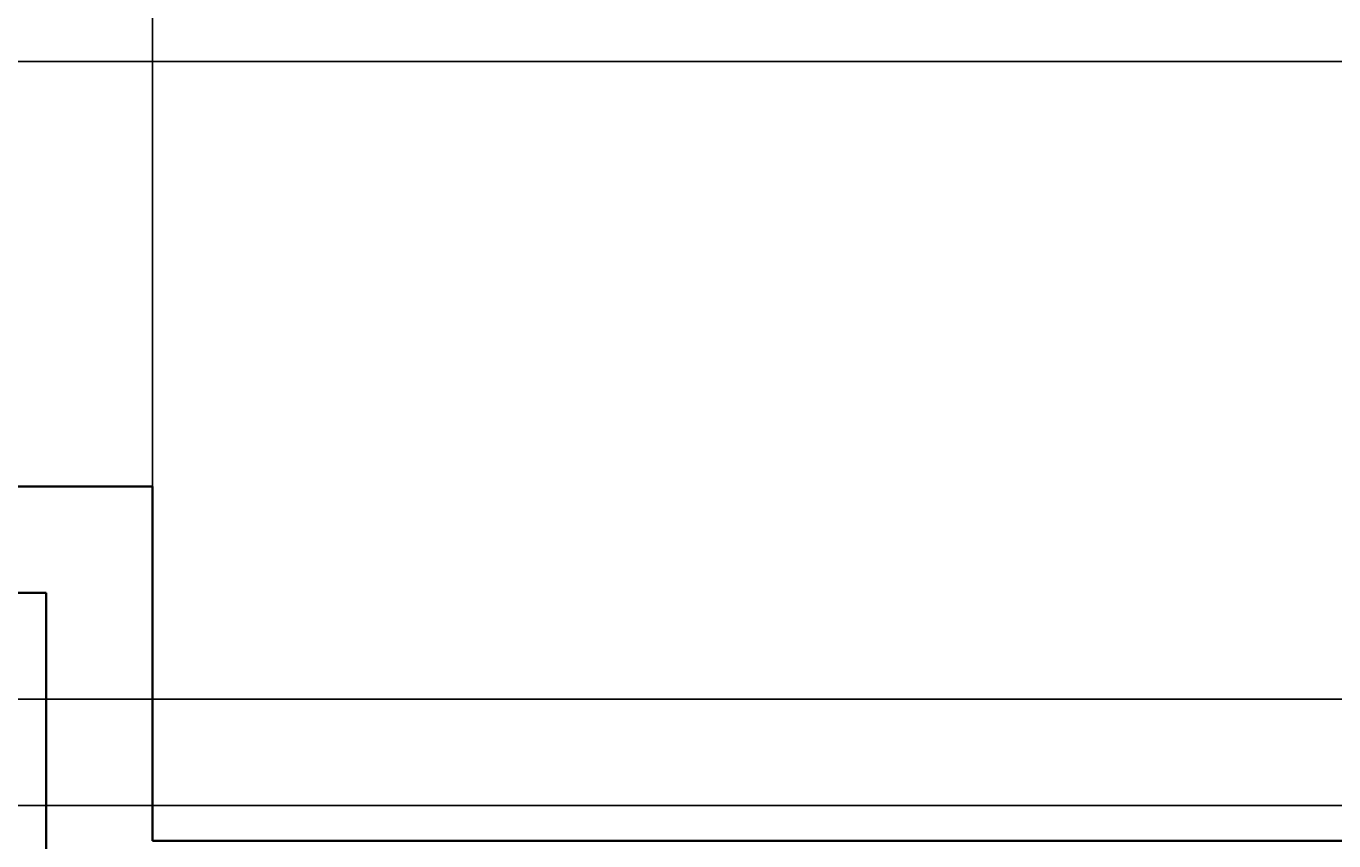
# Model space of a CAD drawing. Units: feet. Extents: x 105 to 1094, y -88 to 588.
# Tile 10 of 59: x 288 to 361, y 204 to 250. Entities that reach past the tile are written whole.
import ezdxf

# ---------------------------------------------------------------- set-up
doc = ezdxf.new("R2010")
doc.units = ezdxf.units.FT
doc.header["$MEASUREMENT"] = 0
doc.layers.add('A-ANNO-DIMS', color=2, linetype='Continuous', lineweight=18)
doc.layers.add('A-WALL', color=7, linetype='Continuous', lineweight=35)
doc.styles.get("Standard").update_dxf_attribs({"font": 'arial.ttf'})
doc.dimstyles.get("Standard").update_dxf_attribs({"dimtxt": 0.18, "dimasz": 0.18, "dimexe": 0.18, "dimexo": 0.0625, "dimgap": 0.09, "dimtad": 0, "dimtih": 1, "dimtoh": 1, "dimdec": 4, "dimzin": 0, "dimdsep": 46, "dimtxsty": 'Standard', "dimcen": 0.09, "dimadec": 0, "dimazin": 0, "dimtfac": 1, "dimtdec": 4, "dimtofl": 0, "dimtmove": 0, "dimatfit": 3, "dimfxl": 1, "dimtolj": 1, "dimtzin": 0, "dimarcsym": 0})

# ---------------------------------------------------------------- blocks, each defined once
blk = doc.blocks.new('*D20')
at = {"layer": 'A-ANNO-DIMS', "color": 0, "lineweight": -2, "transparency": 16777216}
for p, q in [((150.688, 276.019), (150.688, -88.149)), ((1048.688, 276.019), (1048.688, -88.149)), ((150.868, -87.969), (599.399, -87.969)), ((1048.508, -87.969), (599.977, -87.969))]:
    blk.add_line(p, q, dxfattribs=at)
at = {"layer": 'A-ANNO-DIMS', "color": 0, "transparency": 16777216}
for points in [[(150.868, -87.939), (150.868, -87.999), (150.688, -87.969)], [(1048.508, -87.939), (1048.508, -87.999), (1048.688, -87.969)]]:
    blk.add_solid(points, dxfattribs=at)
at = {"layer": 'Defpoints', "color": 0, "transparency": 16777216}
for p in [(150.688, 276.081), (1048.688, 276.081), (1048.688, -87.969)]:
    blk.add_point(p, dxfattribs=at)
at = {"layer": 'A-ANNO-DIMS', "color": 0, "transparency": 16777216, "insert": (599.688, -87.969), "char_height": 0.18, "attachment_point": 5}
blk.add_mtext('\\A1;898', dxfattribs=at)
blk = doc.blocks.new('*D21')
at = {"layer": 'A-ANNO-DIMS', "color": 0, "lineweight": -2, "transparency": 16777216}
for p, q in [((849.626, 543.081), (105.458, 543.081)), ((105.638, 542.901), (105.638, 250.263)), ((105.638, -42.739), (105.638, 249.899)), ((849.626, -42.919), (105.458, -42.919))]:
    blk.add_line(p, q, dxfattribs=at)
at = {"layer": 'A-ANNO-DIMS', "color": 0, "transparency": 16777216}
for points in [[(105.608, 542.901), (105.668, 542.901), (105.638, 543.081)], [(105.608, -42.739), (105.668, -42.739), (105.638, -42.919)]]:
    blk.add_solid(points, dxfattribs=at)
at = {"layer": 'Defpoints', "color": 0, "transparency": 16777216}
for p in [(105.638, 543.081), (849.688, 543.081), (849.688, -42.919)]:
    blk.add_point(p, dxfattribs=at)
at = {"layer": 'A-ANNO-DIMS', "color": 0, "transparency": 16777216, "insert": (105.638, 250.081), "char_height": 0.18, "attachment_point": 5}
blk.add_mtext('\\A1;586', dxfattribs=at)
blk = doc.blocks.new('*D36')
at = {"layer": 'A-ANNO-DIMS', "color": 0, "lineweight": -2, "transparency": 16777216}
for p, q in [((547.235, 248.081), (105.458, 248.081)), ((105.638, 247.901), (105.638, 230.263)), ((105.638, 212.261), (105.638, 229.899)), ((546.626, 212.081), (105.458, 212.081))]:
    blk.add_line(p, q, dxfattribs=at)
at = {"layer": 'A-ANNO-DIMS', "color": 0, "transparency": 16777216}
for points in [[(105.608, 247.901), (105.668, 247.901), (105.638, 248.081)], [(105.608, 212.261), (105.668, 212.261), (105.638, 212.081)]]:
    blk.add_solid(points, dxfattribs=at)
at = {"layer": 'Defpoints', "color": 0, "transparency": 16777216}
for p in [(105.638, 248.081), (547.298, 248.081), (546.688, 212.081)]:
    blk.add_point(p, dxfattribs=at)
at = {"layer": 'A-ANNO-DIMS', "color": 0, "transparency": 16777216, "insert": (105.638, 230.081), "char_height": 0.18, "attachment_point": 5}
blk.add_mtext('\\A1;36', dxfattribs=at)
blk = doc.blocks.new('*D38')
at = {"layer": 'A-ANNO-DIMS', "color": 0, "lineweight": -2, "transparency": 16777216}
for p, q in [((150.688, 224.144), (150.688, 588.311)), ((150.868, 588.131), (222.408, 588.131)), ((294.508, 588.131), (222.968, 588.131)), ((294.688, 224.144), (294.688, 588.311))]:
    blk.add_line(p, q, dxfattribs=at)
at = {"layer": 'A-ANNO-DIMS', "color": 0, "transparency": 16777216}
for points in [[(150.868, 588.161), (150.868, 588.101), (150.688, 588.131)], [(294.508, 588.161), (294.508, 588.101), (294.688, 588.131)]]:
    blk.add_solid(points, dxfattribs=at)
at = {"layer": 'Defpoints', "color": 0, "transparency": 16777216}
for p in [(294.688, 588.131), (150.688, 224.081), (294.688, 224.081)]:
    blk.add_point(p, dxfattribs=at)
at = {"layer": 'A-ANNO-DIMS', "color": 0, "transparency": 16777216, "insert": (222.688, 588.131), "char_height": 0.18, "attachment_point": 5}
blk.add_mtext('\\A1;144', dxfattribs=at)
blk = doc.blocks.new('*D39')
at = {"layer": 'A-ANNO-DIMS', "color": 0, "lineweight": -2, "transparency": 16777216}
for p, q in [((294.688, 204.144), (294.688, 588.311)), ((294.868, 588.131), (332.47, 588.131)), ((370.508, 588.131), (332.906, 588.131)), ((370.688, 204.144), (370.688, 588.311))]:
    blk.add_line(p, q, dxfattribs=at)
at = {"layer": 'A-ANNO-DIMS', "color": 0, "transparency": 16777216}
for points in [[(294.868, 588.161), (294.868, 588.101), (294.688, 588.131)], [(370.508, 588.161), (370.508, 588.101), (370.688, 588.131)]]:
    blk.add_solid(points, dxfattribs=at)
at = {"layer": 'Defpoints', "color": 0, "transparency": 16777216}
for p in [(370.688, 588.131), (294.688, 204.081), (370.688, 204.081)]:
    blk.add_point(p, dxfattribs=at)
at = {"layer": 'A-ANNO-DIMS', "color": 0, "transparency": 16777216, "insert": (332.688, 588.131), "char_height": 0.18, "attachment_point": 5}
blk.add_mtext('\\A1;76', dxfattribs=at)
blk = doc.blocks.new('*D46')
at = {"layer": 'A-ANNO-DIMS', "color": 0, "lineweight": -2, "transparency": 16777216}
for p, q in [((580.626, 206.081), (105.458, 206.081)), ((105.638, 205.901), (105.638, 173.263)), ((105.638, 140.261), (105.638, 172.899)), ((580.626, 140.081), (105.458, 140.081))]:
    blk.add_line(p, q, dxfattribs=at)
at = {"layer": 'A-ANNO-DIMS', "color": 0, "transparency": 16777216}
for points in [[(105.608, 205.901), (105.668, 205.901), (105.638, 206.081)], [(105.608, 140.261), (105.668, 140.261), (105.638, 140.081)]]:
    blk.add_solid(points, dxfattribs=at)
at = {"layer": 'Defpoints', "color": 0, "transparency": 16777216}
for p in [(580.688, 206.081), (105.638, 140.081), (580.688, 140.081)]:
    blk.add_point(p, dxfattribs=at)
at = {"layer": 'A-ANNO-DIMS', "color": 0, "transparency": 16777216, "insert": (105.638, 173.081), "char_height": 0.18, "attachment_point": 5}
blk.add_mtext('\\A1;66', dxfattribs=at)

msp = doc.modelspace()

# ---------------------------------------------------------------- linework, layer by layer
at = {"layer": 'A-WALL'}
for p, q in [((294.6883, 224.0812), (150.6883, 224.0812)), ((294.6883, 224.0812), (294.6883, 204.0812)), ((288.6883, 218.0812), (156.6883, 218.0812)), ((288.6883, 218.0812), (288.6883, 180.0812)), ((370.6883, 204.0812), (294.6883, 204.0812))]:
    msp.add_line(p, q, dxfattribs=at)

# ---------------------------------------------------------------- dimensions: what is measured, and where the dimension line sits
at = {"layer": 'A-ANNO-DIMS'}
for base, p1, p2, picture, middle in [((294.6883, 588.1312), (150.6883, 224.0812), (294.6883, 224.0812), '*D38', (222.6883, 588.1312)), ((370.6883, 588.1312), (294.6883, 204.0812), (370.6883, 204.0812), '*D39', (332.6883, 588.1312)), ((1048.6883, -87.9688), (150.6883, 276.0812), (1048.6883, 276.0812), '*D20', (599.6883, -87.9688))]:
    dim = msp.add_linear_dim(base=base, p1=p1, p2=p2, dimstyle='Standard', override={"dimdec": 0, "dimlfac": 1, "dimrnd": 0, "dimzin": 0, "dimdsep": 46, "dimlunit": 2}, dxfattribs=at)
    dim.commit()
    dim.dimension.update_dxf_attribs({"geometry": picture, "text_midpoint": middle})
for base, p1, p2, picture, middle in [((105.6383, 543.0812), (849.6883, -42.9188), (849.6883, 543.0812), '*D21', (105.6383, 250.0812)), ((105.6383, 248.0812), (546.6883, 212.0812), (547.2975, 248.0812), '*D36', (105.6383, 230.0812)), ((105.6383, 140.0812), (580.6883, 206.0812), (580.6883, 140.0812), '*D46', (105.6383, 173.0812))]:
    dim = msp.add_linear_dim(base=base, p1=p1, p2=p2, angle=90, dimstyle='Standard', override={"dimdec": 0, "dimlfac": 1, "dimrnd": 0, "dimzin": 0, "dimdsep": 46, "dimlunit": 2}, dxfattribs=at)
    dim.commit()
    dim.dimension.update_dxf_attribs({"geometry": picture, "text_midpoint": middle})

doc.saveas('drawing.dxf')
